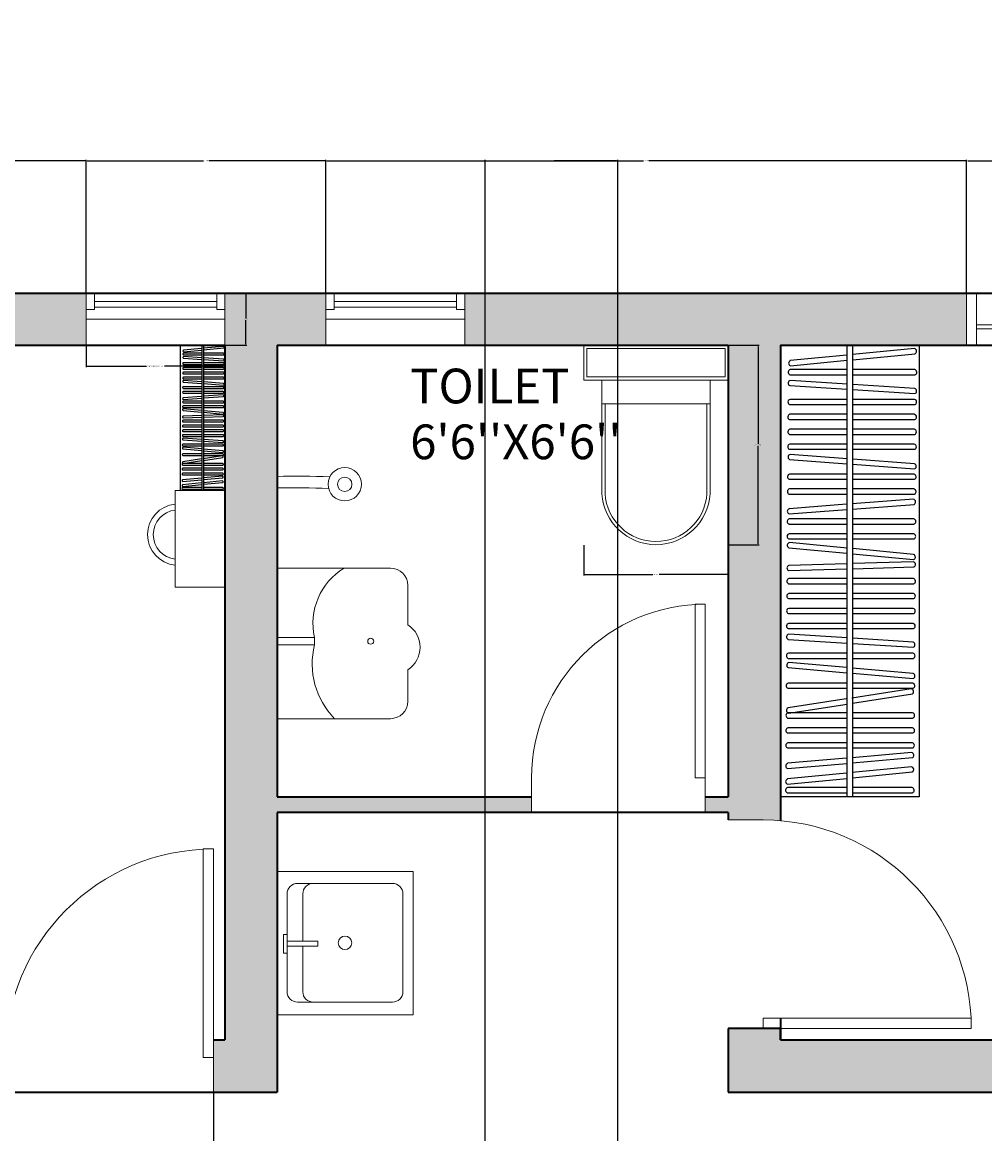
# Model space of a CAD drawing. Units: inches. Extents: x 1789 to 2841, y 3180 to 3702.
# Tile 6 of 14: x 2041 to 2208, y 3510 to 3702. Entities that reach past the tile are written whole.
import ezdxf

# ---------------------------------------------------------------- set-up
doc = ezdxf.new("R2010")
doc.units = ezdxf.units.IN
doc.header["$MEASUREMENT"] = 0
for name, color, linetype, lineweight in [('A-ANNO-DIMS', 2, 'Continuous', 18), ('A-AREA-IDEN', 7, 'Continuous', 18), ('A-FLOR-CASE', 34, 'Continuous', 25), ('A-FLOR-FIXT', 9, 'Continuous', 18), ('A-WALL', 40, 'Continuous', 35), ('A-WALL-PATT', 252, 'Continuous', 13), ('DORS', 70, 'Continuous', 18), ('FURNITURE', 34, 'Continuous', 18), ('WINDOWS', 130, 'Continuous', 18)]:
    doc.layers.add(name, color=color, linetype=linetype, lineweight=lineweight)
doc.styles.get("Standard").update_dxf_attribs({"font": 'arial.ttf'})
doc.dimstyles.get("Standard").update_dxf_attribs({"dimtxt": 0.18, "dimasz": 0.18, "dimexe": 0.18, "dimexo": 0.0625, "dimgap": 0.09, "dimtad": 0, "dimtih": 1, "dimtoh": 1, "dimdec": 0, "dimzin": 0, "dimdsep": 46, "dimlunit": 3, "dimtxsty": 'Standard', "dimcen": 0.09, "dimadec": 0, "dimazin": 0, "dimtfac": 1, "dimtdec": 0, "dimtofl": 0, "dimtmove": 0, "dimatfit": 3, "dimfxl": 1, "dimtolj": 1, "dimtzin": 0, "dimarcsym": 0})

# ---------------------------------------------------------------- blocks, each defined once
blk = doc.blocks.new('HY')
for p, q in [((2053.67, 3653.75), (2074.8, 3653.75)), ((2053.67, 3652.75), (2074.8, 3652.75)), ((2052.23, 3650.66), (2076.23, 3650.66))]:
    blk.add_line(p, q)
for points in [[(2076.23, 3646.16), (2052.23, 3646.16), (2052.23, 3655.16), (2076.23, 3655.16)], [(2052.23, 3655.16), (2053.67, 3655.16), (2053.67, 3652.35), (2052.23, 3652.35)], [(2076.23, 3655.16), (2074.8, 3655.16), (2074.8, 3652.35), (2076.23, 3652.35)]]:
    blk.add_lwpolyline(points, close=True)
blk = doc.blocks.new('HYJ')
for p, q in [((2236.02, 3650.77), (2262.74, 3650.77)), ((2206.12, 3649.67), (2234.3, 3649.67)), ((2206.12, 3649), (2234.3, 3649)), ((2236.02, 3650.11), (2262.74, 3650.11))]:
    blk.add_line(p, q)
for points in [[(2204.43, 3646.16), (2264.43, 3646.16), (2264.43, 3655.16), (2204.43, 3655.16)], [(2204.43, 3655.16), (2206.12, 3655.16), (2206.12, 3646.16), (2204.43, 3646.16)], [(2264.43, 3655.16), (2262.74, 3655.16), (2262.74, 3646.16), (2264.43, 3646.16)], [(2235.16, 3650.77), (2236.02, 3650.77), (2236.02, 3649.67), (2235.16, 3649.67)], [(2234.3, 3649.67), (2235.16, 3649.67), (2235.16, 3648.56), (2234.3, 3648.56)]]:
    blk.add_lwpolyline(points, close=True)
blk = doc.blocks.new('CUBOARD')
for p, q in [((2183.73, 3646.16), (2183.73, 3568.16)), ((2184.71, 3646.16), (2184.71, 3568.16))]:
    blk.add_line(p, q)
blk.add_lwpolyline([(2172.23, 3646.16), (2196.23, 3646.16), (2196.23, 3568.16), (2172.23, 3568.16)], close=True)
for points in [[(2183.69, 3644.46), (2173.95, 3643.51)], [(2195.39, 3645.6), (2184.67, 3644.55)], [(2184.76, 3643.66), (2195.54, 3644.71)], [(2195.78, 3645.16), (2195.78, 3645.18)], [(2173.97, 3642.61), (2183.78, 3643.57)], [(2173.86, 3641.08), (2183.73, 3641.08)], [(2183.73, 3641.98), (2173.93, 3641.98)], [(2195.47, 3641.98), (2184.71, 3641.98)], [(2184.71, 3641.08), (2195.53, 3641.08)], [(2195.82, 3641.5), (2195.82, 3641.53)], [(2173.84, 3639.19), (2183.7, 3638.57)], [(2183.76, 3639.46), (2173.96, 3640.08)], [(2195.45, 3638.71), (2184.74, 3639.4)], [(2183.73, 3636.82), (2173.9, 3636.82)], [(2184.68, 3638.5), (2195.46, 3637.81)], [(2195.43, 3636.82), (2184.71, 3636.82)], [(2195.77, 3638.22), (2195.78, 3638.24)], [(2173.83, 3635.92), (2183.73, 3635.92)], [(2184.71, 3635.92), (2195.5, 3635.92)], [(2195.78, 3636.35), (2195.78, 3636.37)], [(2173.81, 3633.34), (2183.73, 3633.34)], [(2183.73, 3634.24), (2173.88, 3634.24)], [(2195.42, 3634.24), (2184.71, 3634.24)], [(2184.71, 3633.34), (2195.48, 3633.34)], [(2195.77, 3633.77), (2195.77, 3633.79)], [(2183.73, 3631.66), (2173.86, 3631.66)], [(2195.4, 3631.66), (2184.71, 3631.66)], [(2195.75, 3631.19), (2195.75, 3631.21)], [(2173.8, 3630.76), (2183.73, 3630.76)], [(2183.73, 3629.08), (2173.85, 3629.08)], [(2184.71, 3630.76), (2195.47, 3630.76)], [(2195.38, 3629.08), (2184.71, 3629.08)], [(2173.78, 3628.19), (2183.73, 3628.19)], [(2183.8, 3626.57), (2173.93, 3627.31)], [(2184.71, 3628.19), (2195.45, 3628.19)], [(2195.73, 3628.61), (2195.73, 3628.63)], [(2173.79, 3626.43), (2183.74, 3625.68)], [(2184.71, 3625.61), (2195.4, 3624.81)], [(2195.4, 3625.7), (2184.78, 3626.5)], [(2195.72, 3625.21), (2195.72, 3625.23)], [(2183.73, 3623.92), (2173.81, 3623.92)], [(2195.35, 3623.92), (2184.71, 3623.92)], [(2195.7, 3623.45), (2195.7, 3623.48)], [(2173.75, 3623.03), (2183.73, 3623.03)], [(2183.73, 3621.34), (2173.8, 3621.34)], [(2184.71, 3623.03), (2195.42, 3623.03)], [(2195.33, 3621.34), (2184.71, 3621.34)], [(2173.73, 3620.45), (2183.73, 3620.45)], [(2195.22, 3619.57), (2184.65, 3618.76)], [(2184.71, 3620.45), (2195.4, 3620.45)], [(2195.68, 3620.87), (2195.68, 3620.9)], [(2183.67, 3618.69), (2173.75, 3617.93)], [(2173.75, 3617.03), (2183.74, 3617.8)], [(2184.71, 3617.87), (2195.35, 3618.68)], [(2195.6, 3619.13), (2195.6, 3619.15)], [(2183.73, 3616.19), (2173.77, 3616.19)], [(2195.3, 3616.19), (2184.71, 3616.19)], [(2195.65, 3615.71), (2195.65, 3615.74)], [(2173.7, 3615.29), (2183.73, 3615.29)], [(2184.71, 3615.29), (2195.37, 3615.29)], [(2173.68, 3612.71), (2183.73, 3612.71)], [(2183.73, 3613.61), (2173.75, 3613.61)], [(2183.78, 3611.12), (2173.82, 3612.07)], [(2195.28, 3613.61), (2184.71, 3613.61)], [(2184.71, 3612.71), (2195.35, 3612.71)], [(2195.63, 3613.14), (2195.63, 3613.16)], [(2173.67, 3611.18), (2183.69, 3610.23)], [(2184.67, 3610.14), (2195.24, 3609.13)], [(2195.26, 3610.03), (2184.75, 3611.03)], [(2183.72, 3608.42), (2173.71, 3608.13)], [(2195.23, 3608.76), (2184.7, 3608.45)], [(2195.56, 3609.53), (2195.57, 3609.55)], [(2195.6, 3608.3), (2195.6, 3608.32)], [(2173.66, 3607.23), (2183.75, 3607.53)], [(2184.73, 3607.55), (2195.33, 3607.87)], [(2173.63, 3604.98), (2183.73, 3604.98)], [(2183.73, 3605.87), (2173.7, 3605.87)], [(2195.23, 3605.87), (2184.71, 3605.87)], [(2184.71, 3604.98), (2195.3, 3604.98)], [(2195.58, 3605.4), (2195.58, 3605.42)], [(2173.61, 3602.4), (2183.73, 3602.4)], [(2183.73, 3603.29), (2173.68, 3603.29)], [(2195.22, 3603.29), (2184.71, 3603.29)], [(2184.71, 3602.4), (2195.28, 3602.4)], [(2195.57, 3602.82), (2195.57, 3602.84)], [(2183.73, 3600.71), (2173.67, 3600.71)], [(2195.2, 3600.71), (2184.71, 3600.71)], [(2195.55, 3600.24), (2195.55, 3600.27)], [(2173.6, 3599.82), (2183.73, 3599.82)], [(2184.71, 3599.82), (2195.27, 3599.82)], [(2173.58, 3597.24), (2183.73, 3597.24)], [(2183.73, 3598.13), (2173.65, 3598.13)], [(2195.18, 3598.13), (2184.71, 3598.13)], [(2184.71, 3597.24), (2195.25, 3597.24)], [(2195.53, 3597.66), (2195.53, 3597.69)], [(2173.56, 3595.36), (2183.71, 3594.72)], [(2183.77, 3595.62), (2173.68, 3596.25)], [(2184.69, 3594.66), (2195.19, 3594)], [(2195.18, 3594.9), (2184.74, 3595.55)], [(2183.73, 3592.98), (2173.62, 3592.98)], [(2195.15, 3592.98), (2184.71, 3592.98)], [(2195.5, 3594.4), (2195.5, 3594.43)], [(2195.5, 3592.5), (2195.5, 3592.53)], [(2173.55, 3592.08), (2183.73, 3592.08)], [(2183.73, 3590.49), (2173.72, 3591.37)], [(2184.71, 3592.08), (2195.22, 3592.08)], [(2173.57, 3590.49), (2183.74, 3589.59)], [(2195.17, 3589.47), (2184.71, 3590.4)], [(2184.71, 3589.5), (2195.16, 3588.58)], [(2195.48, 3588.97), (2195.48, 3589)], [(2173.51, 3586.92), (2183.73, 3586.92)], [(2183.73, 3587.82), (2173.58, 3587.82)], [(2194.84, 3586.83), (2184.58, 3585.23)], [(2195.12, 3587.82), (2184.71, 3587.82)], [(2184.71, 3586.92), (2195.19, 3586.92)], [(2195.47, 3587.35), (2195.47, 3587.37)], [(2183.61, 3585.08), (2173.56, 3583.51)], [(2184.71, 3584.34), (2195.04, 3585.95)], [(2195.26, 3586.41), (2195.25, 3586.44)], [(2173.63, 3582.62), (2183.75, 3584.19)], [(2173.48, 3581.77), (2183.73, 3581.77)], [(2183.73, 3582.66), (2173.55, 3582.66)], [(2195.08, 3582.66), (2184.71, 3582.66)], [(2184.71, 3581.77), (2195.15, 3581.77)], [(2195.43, 3582.19), (2195.43, 3582.21)], [(2173.46, 3579.19), (2183.73, 3579.19)], [(2183.73, 3580.08), (2173.53, 3580.08)], [(2195.07, 3580.08), (2184.71, 3580.08)], [(2184.71, 3579.19), (2195.14, 3579.19)], [(2195.42, 3579.61), (2195.42, 3579.63)], [(2183.73, 3577.5), (2173.52, 3577.5)], [(2195.05, 3577.5), (2184.71, 3577.5)], [(2173.45, 3576.61), (2183.73, 3576.61)], [(2194.92, 3575.81), (2184.64, 3574.92)], [(2184.71, 3576.61), (2195.12, 3576.61)], [(2195.31, 3575.37), (2195.31, 3575.4)], [(2195.4, 3577.03), (2195.4, 3577.05)], [(2183.66, 3574.84), (2173.46, 3573.95)], [(2173.47, 3573.05), (2183.74, 3573.94)], [(2194.88, 3573.34), (2184.63, 3572.34)], [(2184.71, 3574.03), (2195.06, 3574.93)], [(2183.65, 3572.24), (2173.45, 3571.25)], [(2184.71, 3571.45), (2195.04, 3572.46)], [(2195.28, 3572.91), (2195.27, 3572.93)], [(2173.47, 3570.35), (2183.74, 3571.35)], [(2183.73, 3569.77), (2173.47, 3569.77)], [(2195, 3569.77), (2184.71, 3569.77)], [(2173.4, 3568.87), (2183.73, 3568.87)], [(2184.71, 3568.87), (2195.07, 3568.87)], [(2195.35, 3569.29), (2195.35, 3569.32)]]:
    blk.add_lwpolyline(points)
for centre, start, end in [((2195.31, 3645.13), 7.0195, 80.386), ((2195.31, 3645.13), 299.464, 4.1032), ((2174.12, 3643.06), 110.7367, 251.6587), ((2174.06, 3641.52), 105.1753, 246.0974), ((2195.34, 3641.52), 1.4582, 74.8247), ((2195.34, 3641.52), 293.9026, 358.5418), ((2174.06, 3639.62), 101.5232, 242.4452), ((2195.3, 3638.26), 357.8061, 71.1726), ((2174.02, 3636.36), 105.1753, 246.0974), ((2195.31, 3636.36), 1.4582, 74.8247), ((2195.3, 3638.26), 290.2505, 354.8897), ((2195.31, 3636.36), 293.9026, 358.5418), ((2174.01, 3633.78), 105.1753, 246.0974), ((2195.29, 3633.78), 1.4582, 74.8247), ((2195.29, 3633.78), 293.9026, 358.5418), ((2173.99, 3631.2), 105.1753, 246.0974), ((2195.27, 3631.2), 1.4582, 74.8247), ((2195.27, 3631.2), 293.9026, 358.5418), ((2173.97, 3628.62), 105.1753, 246.0974), ((2195.26, 3628.62), 1.4582, 74.8247), ((2174.02, 3626.85), 100.888, 241.81), ((2195.26, 3628.62), 293.9026, 358.5418), ((2195.24, 3625.25), 357.1709, 70.5374), ((2195.24, 3625.25), 289.6153, 354.2545), ((2173.94, 3623.46), 105.1753, 246.0974), ((2195.22, 3623.46), 1.4582, 74.8247), ((2195.22, 3623.46), 293.9026, 358.5418), ((2173.92, 3620.88), 105.1753, 246.0974), ((2195.21, 3620.88), 1.4582, 74.8247), ((2195.13, 3619.1), 5.8369, 79.2034), ((2195.21, 3620.88), 293.9026, 358.5418), ((2173.9, 3617.48), 109.5541, 250.4761), ((2195.13, 3619.1), 298.2814, 2.9206), ((2173.89, 3615.73), 105.1753, 246.0974), ((2195.17, 3615.73), 1.4582, 74.8247), ((2195.17, 3615.73), 293.9026, 358.5418), ((2173.87, 3613.15), 105.1753, 246.0974), ((2173.9, 3611.6), 99.7479, 240.6699), ((2195.16, 3613.15), 1.4582, 74.8247), ((2195.16, 3613.15), 293.9026, 358.5418), ((2195.09, 3609.58), 356.0307, 69.3973), ((2173.84, 3607.67), 106.858, 247.78), ((2195.12, 3608.3), 3.1408, 76.5073), ((2195.09, 3609.58), 288.4752, 353.1144), ((2195.12, 3608.3), 295.5853, 0.2245), ((2173.82, 3605.41), 105.1753, 246.0974), ((2195.11, 3605.41), 1.4582, 74.8247), ((2195.11, 3605.41), 293.9026, 358.5418), ((2173.81, 3602.83), 105.1753, 246.0974), ((2195.09, 3602.83), 1.4582, 74.8247), ((2195.09, 3602.83), 293.9026, 358.5418), ((2173.79, 3600.25), 105.1753, 246.0974), ((2195.08, 3600.25), 1.4582, 74.8247), ((2195.08, 3600.25), 293.9026, 358.5418), ((2173.77, 3597.67), 105.1753, 246.0974), ((2195.06, 3597.67), 1.4582, 74.8247), ((2195.06, 3597.67), 293.9026, 358.5418), ((2173.78, 3595.78), 101.566, 242.4881), ((2195.02, 3594.44), 357.8489, 71.2154), ((2173.74, 3592.52), 105.1753, 246.0974), ((2195.03, 3592.52), 1.4582, 74.8247), ((2195.02, 3594.44), 290.2933, 354.9325), ((2173.8, 3590.9), 100.1162, 241.0382), ((2195.03, 3592.52), 293.9026, 358.5418), ((2195.01, 3589.03), 288.8435, 353.4827), ((2195.01, 3589.03), 356.399, 69.7655), ((2173.71, 3587.36), 105.1753, 246.0974), ((2194.79, 3586.35), 10.3063, 83.6728), ((2194.99, 3587.36), 1.4582, 74.8247), ((2194.99, 3587.36), 293.9026, 358.5418), ((2194.79, 3586.35), 302.7507, 7.3899), ((2173.75, 3583.08), 114.0234, 254.9455), ((2173.67, 3582.2), 105.1753, 246.0974), ((2194.96, 3582.2), 1.4582, 74.8247), ((2194.96, 3582.2), 293.9026, 358.5418), ((2173.66, 3579.62), 105.1753, 246.0974), ((2194.94, 3579.62), 1.4582, 74.8247), ((2194.94, 3579.62), 293.9026, 358.5418), ((2173.64, 3577.04), 105.1753, 246.0974), ((2194.93, 3577.04), 1.4582, 74.8247), ((2194.83, 3575.34), 6.4142, 79.7807), ((2194.83, 3575.34), 298.8587, 3.4979), ((2194.93, 3577.04), 293.9026, 358.5418), ((2173.63, 3573.5), 110.1314, 251.0534), ((2194.8, 3572.87), 7.0476, 80.4142), ((2194.8, 3572.87), 299.4921, 4.1313), ((2173.59, 3569.31), 105.1753, 246.0974), ((2173.62, 3570.8), 110.7648, 251.6868), ((2194.88, 3569.31), 1.4582, 74.8247), ((2194.88, 3569.31), 293.9026, 358.5418)]:
    blk.add_arc(centre, 0.476, start, end)
blk = doc.blocks.new('GT')
for p, q in [((2141.38, 3640.15), (2141.38, 3620.49)), ((2160.08, 3640.15), (2160.08, 3620.49)), ((2141.38, 3636.04), (2160.08, 3636.04)), ((2141.93, 3636.04), (2141.93, 3620.49)), ((2159.53, 3636.04), (2159.53, 3620.49))]:
    blk.add_line(p, q)
for points in [[(2163.23, 3646.16), (2138.23, 3646.16), (2138.23, 3640.15), (2163.23, 3640.15)], [(2162.68, 3645.61), (2138.78, 3645.61), (2138.78, 3640.7), (2162.68, 3640.7)]]:
    blk.add_lwpolyline(points, close=True)
for radius in [9.37, 8.82]:
    blk.add_arc((2150.73, 3621.09), radius, 183.6546, 356.3454)
blk = doc.blocks.new('KIKI')
blk.add_lwpolyline([(2076.23, 3621.09), (2067.63, 3621.09), (2067.63, 3604.37), (2076.23, 3604.37)], close=True)
for radius, start, end in [(5.28, 95.3029, 264.6971), (4.28, 96.5454, 263.4546)]:
    blk.add_arc((2068.12, 3613.45), radius, start, end)
blk = doc.blocks.new('*U9')
for p, q in [((0, 0), (0, -6)), ((36, 0), (36, -6))]:
    blk.add_line(p, q)
blk.add_lwpolyline([(0, 0), (0, 36), (1.75, 36), (1.75, 0)], close=True)
blk.add_arc((0, 0), 36, 0, 90)
blk = doc.blocks.new('*U10')
for p, q in [((0, 0), (0, -6)), ((30, 0), (30, -6))]:
    blk.add_line(p, q)
blk.add_lwpolyline([(0, 0), (0, 30), (1.75, 30), (1.75, 0)], close=True)
blk.add_arc((0, 0), 30, 0, 90)
blk = doc.blocks.new('TYTY')
for p, q in [((2104.84, 3607.68), (2085.23, 3607.68)), ((2085.23, 3607.68), (2085.23, 3581.66)), ((2107.84, 3597.9), (2107.84, 3604.68)), ((2107.84, 3584.66), (2107.84, 3590.13)), ((2085.23, 3581.66), (2104.84, 3581.66))]:
    blk.add_line(p, q)
blk.add_lwpolyline([(2085.23, 3595.66), (2091.71, 3595.66), (2091.71, 3594.41), (2085.23, 3594.41)], close=True)
blk.add_circle((2101.42, 3595.04), 0.517)
for centre, radius, start, end in [((2102.58, 3598.14), 11.14, 121.1396, 192.8397), ((2104.84, 3604.68), 3, 0, 90), ((2105.34, 3594.01), 4.62, 302.7804, 57.2196), ((2104.89, 3591.14), 13.58, 166.0641, 224.2681), ((2104.84, 3584.66), 3, 270, 0)]:
    blk.add_arc(centre, radius, start, end)
blk = doc.blocks.new('SINK')
for points in [[(2247.56, 3305.33), (2275.07, 3305.33), (2275.07, 3279.16), (2247.56, 3279.16)], [(2260.91, 3287.01), (2261.87, 3287.01), (2261.87, 3281.09), (2260.91, 3281.09)], [(2259.67, 3281.09), (2263.21, 3281.09), (2263.21, 3280.41), (2259.67, 3280.41)]]:
    blk.add_lwpolyline(points, close=True)
blk.add_lwpolyline([(2251.84, 3281.09), (2270.63, 3281.09, 0.414214), (2272.63, 3283.09), (2272.63, 3301.33, 0.414214), (2270.63, 3303.33), (2251.84, 3303.33, 0.414214), (2249.84, 3301.33), (2249.84, 3283.09, 0.414214)], format="xyb", close=True)
for points in [[(2249.84, 3301.33), (2249.84, 3286.11, 0.414214), (2251.84, 3284.11), (2260.91, 3284.11)], [(2261.87, 3284.11), (2270.63, 3284.11, 0.414214), (2272.63, 3286.11), (2272.63, 3301.33)]]:
    blk.add_lwpolyline(points, format="xyb")
blk.add_circle((2261.24, 3292.21), 1.3)
blk = doc.blocks.new('SOUW')
for radius in [2.88, 1.24]:
    blk.add_circle((2096.93, 3622.15), radius)
for radius, start in [(130.14, 87.3378), (128.14, 87.3891)]:
    blk.add_arc((2088.3, 3493.42), radius, start, 91.3578)
blk = doc.blocks.new('*D29')
at = {"layer": 'A-ANNO-DIMS', "color": 0, "lineweight": -2, "transparency": 16777216}
for p, q in [((2052.23, 3646.1), (2052.23, 3642.38)), ((2076.23, 3646.1), (2076.23, 3642.38)), ((2052.41, 3642.56), (2062.67, 3642.56)), ((2076.05, 3642.56), (2065.79, 3642.56))]:
    blk.add_line(p, q, dxfattribs=at)
at = {"layer": 'A-ANNO-DIMS', "color": 0, "transparency": 16777216}
for points in [[(2052.41, 3642.59), (2052.41, 3642.53), (2052.23, 3642.56)], [(2076.05, 3642.59), (2076.05, 3642.53), (2076.23, 3642.56)]]:
    blk.add_solid(points, dxfattribs=at)
at = {"layer": 'Defpoints', "color": 0, "transparency": 16777216}
for p in [(2052.23, 3646.16), (2076.23, 3646.16), (2076.23, 3642.56)]:
    blk.add_point(p, dxfattribs=at)
at = {"layer": 'A-ANNO-DIMS', "color": 0, "transparency": 16777216, "insert": (2064.23, 3642.56), "char_height": 0.18, "attachment_point": 5}
blk.add_mtext('\\A1;SMALL WINDOW 24 TYP.', dxfattribs=at)
blk = doc.blocks.new('*D30')
at = {"layer": 'A-ANNO-DIMS', "color": 0, "lineweight": -2, "transparency": 16777216}
for p, q in [((2076.3, 3655.16), (2080.01, 3655.16)), ((2079.83, 3654.98), (2079.83, 3650.84)), ((2079.83, 3646.34), (2079.83, 3650.48)), ((2076.3, 3646.16), (2080.01, 3646.16))]:
    blk.add_line(p, q, dxfattribs=at)
at = {"layer": 'A-ANNO-DIMS', "color": 0, "transparency": 16777216}
for points in [[(2079.8, 3654.98), (2079.86, 3654.98), (2079.83, 3655.16)], [(2079.8, 3646.34), (2079.86, 3646.34), (2079.83, 3646.16)]]:
    blk.add_solid(points, dxfattribs=at)
at = {"layer": 'Defpoints', "color": 0, "transparency": 16777216}
for p in [(2076.23, 3655.16), (2079.83, 3655.16), (2076.23, 3646.16)]:
    blk.add_point(p, dxfattribs=at)
at = {"layer": 'A-ANNO-DIMS', "color": 0, "transparency": 16777216, "insert": (2079.83, 3650.66), "char_height": 0.18, "attachment_point": 5}
blk.add_mtext('\\A1;9 TYP.', dxfattribs=at)
blk = doc.blocks.new('*D43')
at = {"layer": 'A-ANNO-DIMS', "color": 0, "lineweight": -2, "transparency": 16777216}
for p, q in [((2163.3, 3646.16), (2168.58, 3646.16)), ((2168.4, 3645.98), (2168.4, 3629.12)), ((2168.4, 3611.89), (2168.4, 3628.75)), ((2163.3, 3611.71), (2168.58, 3611.71))]:
    blk.add_line(p, q, dxfattribs=at)
at = {"layer": 'A-ANNO-DIMS', "color": 0, "transparency": 16777216}
for points in [[(2168.37, 3645.98), (2168.43, 3645.98), (2168.4, 3646.16)], [(2168.37, 3611.89), (2168.43, 3611.89), (2168.4, 3611.71)]]:
    blk.add_solid(points, dxfattribs=at)
at = {"layer": 'Defpoints', "color": 0, "transparency": 16777216}
for p in [(2163.23, 3646.16), (2168.4, 3646.16), (2163.23, 3611.71)]:
    blk.add_point(p, dxfattribs=at)
at = {"layer": 'A-ANNO-DIMS', "color": 0, "transparency": 16777216, "insert": (2168.4, 3628.94), "char_height": 0.18, "attachment_point": 5}
blk.add_mtext('\\A1;WC 34 TYP.', dxfattribs=at)
blk = doc.blocks.new('*D44')
at = {"layer": 'A-ANNO-DIMS', "color": 0, "lineweight": -2, "transparency": 16777216}
for p, q in [((2138.23, 3611.65), (2138.23, 3606.37)), ((2163.23, 3611.65), (2163.23, 3606.37)), ((2138.41, 3606.55), (2150.2, 3606.55)), ((2163.05, 3606.55), (2151.26, 3606.55))]:
    blk.add_line(p, q, dxfattribs=at)
at = {"layer": 'A-ANNO-DIMS', "color": 0, "transparency": 16777216}
for points in [[(2138.41, 3606.58), (2138.41, 3606.52), (2138.23, 3606.55)], [(2163.05, 3606.58), (2163.05, 3606.52), (2163.23, 3606.55)]]:
    blk.add_solid(points, dxfattribs=at)
at = {"layer": 'Defpoints', "color": 0, "transparency": 16777216}
for p in [(2138.23, 3611.71), (2163.23, 3611.71), (2163.23, 3606.55)]:
    blk.add_point(p, dxfattribs=at)
at = {"layer": 'A-ANNO-DIMS', "color": 0, "transparency": 16777216, "insert": (2150.73, 3606.55), "char_height": 0.18, "attachment_point": 5}
blk.add_mtext('\\A1;25 TYP.', dxfattribs=at)
blk = doc.blocks.new('*D82')
at = {"layer": 'A-ANNO-DIMS', "color": 0, "lineweight": -2, "transparency": 16777216}
for p, q in [((1959.23, 3655.22), (1959.23, 3678.19)), ((1959.41, 3678.01), (2005.51, 3678.01)), ((2052.05, 3678.01), (2005.95, 3678.01)), ((2052.23, 3655.22), (2052.23, 3678.19))]:
    blk.add_line(p, q, dxfattribs=at)
at = {"layer": 'A-ANNO-DIMS', "color": 0, "transparency": 16777216}
for points in [[(1959.41, 3678.04), (1959.41, 3677.98), (1959.23, 3678.01)], [(2052.05, 3678.04), (2052.05, 3677.98), (2052.23, 3678.01)]]:
    blk.add_solid(points, dxfattribs=at)
at = {"layer": 'Defpoints', "color": 0, "transparency": 16777216}
for p in [(2052.23, 3678.01), (1959.23, 3655.16), (2052.23, 3655.16)]:
    blk.add_point(p, dxfattribs=at)
at = {"layer": 'A-ANNO-DIMS', "color": 0, "transparency": 16777216, "insert": (2005.73, 3678.01), "char_height": 0.18, "attachment_point": 5}
blk.add_mtext('\\A1;93', dxfattribs=at)
blk = doc.blocks.new('*D83')
at = {"layer": 'A-ANNO-DIMS', "color": 0, "lineweight": -2, "transparency": 16777216}
for p, q in [((2052.23, 3655.22), (2052.23, 3678.19)), ((2052.41, 3678.01), (2072.49, 3678.01)), ((2093.5, 3678.01), (2073.42, 3678.01)), ((2093.68, 3655.22), (2093.68, 3678.19))]:
    blk.add_line(p, q, dxfattribs=at)
at = {"layer": 'A-ANNO-DIMS', "color": 0, "transparency": 16777216}
for points in [[(2052.41, 3678.04), (2052.41, 3677.98), (2052.23, 3678.01)], [(2093.5, 3678.04), (2093.5, 3677.98), (2093.68, 3678.01)]]:
    blk.add_solid(points, dxfattribs=at)
at = {"layer": 'Defpoints', "color": 0, "transparency": 16777216}
for p in [(2093.68, 3678.01), (2052.23, 3655.16), (2093.68, 3655.16)]:
    blk.add_point(p, dxfattribs=at)
at = {"layer": 'A-ANNO-DIMS', "color": 0, "transparency": 16777216, "insert": (2072.96, 3678.01), "char_height": 0.18, "attachment_point": 5}
blk.add_mtext('\\A1;41.445', dxfattribs=at)
blk = doc.blocks.new('*D84')
at = {"layer": 'A-ANNO-DIMS', "color": 0, "lineweight": -2, "transparency": 16777216}
for p, q in [((2093.68, 3655.22), (2093.68, 3678.19)), ((2093.86, 3678.01), (2148.6, 3678.01)), ((2204.25, 3678.01), (2149.51, 3678.01)), ((2204.43, 3655.22), (2204.43, 3678.19))]:
    blk.add_line(p, q, dxfattribs=at)
at = {"layer": 'A-ANNO-DIMS', "color": 0, "transparency": 16777216}
for points in [[(2093.86, 3678.04), (2093.86, 3677.98), (2093.68, 3678.01)], [(2204.25, 3678.04), (2204.25, 3677.98), (2204.43, 3678.01)]]:
    blk.add_solid(points, dxfattribs=at)
at = {"layer": 'Defpoints', "color": 0, "transparency": 16777216}
for p in [(2204.43, 3678.01), (2093.68, 3655.16), (2204.43, 3655.16)]:
    blk.add_point(p, dxfattribs=at)
at = {"layer": 'A-ANNO-DIMS', "color": 0, "transparency": 16777216, "insert": (2149.06, 3678.01), "char_height": 0.18, "attachment_point": 5}
blk.add_mtext('\\A1;110.75', dxfattribs=at)
blk = doc.blocks.new('*D85')
at = {"layer": 'A-ANNO-DIMS', "color": 0, "lineweight": -2, "transparency": 16777216}
for p, q in [((2204.43, 3655.22), (2204.43, 3678.19)), ((2204.61, 3678.01), (2264.45, 3678.01)), ((2325.05, 3678.01), (2265.22, 3678.01)), ((2325.23, 3655.22), (2325.23, 3678.19))]:
    blk.add_line(p, q, dxfattribs=at)
at = {"layer": 'A-ANNO-DIMS', "color": 0, "transparency": 16777216}
for points in [[(2204.61, 3678.04), (2204.61, 3677.98), (2204.43, 3678.01)], [(2325.05, 3678.04), (2325.05, 3677.98), (2325.23, 3678.01)]]:
    blk.add_solid(points, dxfattribs=at)
at = {"layer": 'Defpoints', "color": 0, "transparency": 16777216}
for p in [(2325.23, 3678.01), (2204.43, 3655.16), (2325.23, 3655.16)]:
    blk.add_point(p, dxfattribs=at)
at = {"layer": 'A-ANNO-DIMS', "color": 0, "transparency": 16777216, "insert": (2264.83, 3678.01), "char_height": 0.18, "attachment_point": 5}
blk.add_mtext('\\A1;120.8', dxfattribs=at)
blk = doc.blocks.new('*D90')
at = {"layer": 'A-ANNO-DIMS', "color": 0, "lineweight": -2, "transparency": 16777216}
for p, q in [((2038.23, 3517.1), (2038.23, 3180.13)), ((2074.23, 3517.1), (2074.23, 3180.13)), ((2038.41, 3180.31), (2056.01, 3180.31)), ((2074.05, 3180.31), (2056.45, 3180.31))]:
    blk.add_line(p, q, dxfattribs=at)
at = {"layer": 'A-ANNO-DIMS', "color": 0, "transparency": 16777216}
for points in [[(2038.41, 3180.34), (2038.41, 3180.28), (2038.23, 3180.31)], [(2074.05, 3180.34), (2074.05, 3180.28), (2074.23, 3180.31)]]:
    blk.add_solid(points, dxfattribs=at)
at = {"layer": 'Defpoints', "color": 0, "transparency": 16777216}
for p in [(2038.23, 3517.16), (2074.23, 3517.16), (2074.23, 3180.31)]:
    blk.add_point(p, dxfattribs=at)
at = {"layer": 'A-ANNO-DIMS', "color": 0, "transparency": 16777216, "insert": (2056.23, 3180.31), "char_height": 0.18, "attachment_point": 5}
blk.add_mtext('\\A1;36', dxfattribs=at)
blk = doc.blocks.new('*D91')
at = {"layer": 'A-ANNO-DIMS', "color": 0, "lineweight": -2, "transparency": 16777216}
for p, q in [((2121.23, 3385.22), (2121.23, 3678.19)), ((2121.41, 3678.01), (2132.21, 3678.01)), ((2143.93, 3678.01), (2133.14, 3678.01)), ((2144.11, 3385.22), (2144.11, 3678.19))]:
    blk.add_line(p, q, dxfattribs=at)
at = {"layer": 'A-ANNO-DIMS', "color": 0, "transparency": 16777216}
for points in [[(2121.41, 3678.04), (2121.41, 3677.98), (2121.23, 3678.01)], [(2143.93, 3678.04), (2143.93, 3677.98), (2144.11, 3678.01)]]:
    blk.add_solid(points, dxfattribs=at)
at = {"layer": 'Defpoints', "color": 0, "transparency": 16777216}
for p in [(2144.11, 3678.01), (2121.23, 3385.16), (2144.11, 3385.16)]:
    blk.add_point(p, dxfattribs=at)
at = {"layer": 'A-ANNO-DIMS', "color": 0, "transparency": 16777216, "insert": (2132.67, 3678.01), "char_height": 0.18, "attachment_point": 5}
blk.add_mtext('\\A1;22.875', dxfattribs=at)
blk = doc.blocks.new('*D116')
at = {"layer": 'A-ANNO-DIMS', "color": 0, "lineweight": -2, "transparency": 16777216}
for p, q in [((1789.65, 3701.85), (1789.83, 3701.85)), ((1789.83, 3701.85), (1945.65, 3528.3)), ((2205.56, 3238.68), (2205.74, 3238.68)), ((2205.65, 3238.59), (2205.65, 3238.77))]:
    blk.add_line(p, q, dxfattribs=at)
at = {"layer": 'A-ANNO-DIMS', "color": 0, "transparency": 16777216}
blk.add_solid([(1945.67, 3528.32), (1945.62, 3528.28), (1945.77, 3528.16)], dxfattribs=at)
at = {"layer": 'Defpoints', "color": 0, "transparency": 16777216}
for p in [(1945.77, 3528.16), (2205.65, 3238.68)]:
    blk.add_point(p, dxfattribs=at)
at = {"layer": 'A-ANNO-DIMS', "color": 0, "transparency": 16777216, "insert": (1789.28, 3701.85), "char_height": 0.18, "attachment_point": 5}
blk.add_mtext('\\A1;R389', dxfattribs=at)

msp = doc.modelspace()

# ---------------------------------------------------------------- hatches: boundary and pattern name
at = {"layer": 'A-WALL-PATT'}
h = msp.add_hatch(color=256, dxfattribs=at)
h.dxf.hatch_style = 1
h.paths.add_polyline_path([(2052.2333, 3646.1608), (2052.2333, 3655.1608), (1959.2333, 3655.1608), (1959.2333, 3622.3936), (1968.2333, 3622.3936), (1968.2333, 3646.1608)])
h.paths.add_polyline_path([(2163.2333, 3646.1608), (2163.2333, 3640.1475), (2163.2333, 3568.1608), (2159.2333, 3568.1608), (2159.2333, 3565.4274), (2163.2333, 3565.4274), (2163.2333, 3564.1608), (2169.2333, 3564.1608, -0.02086055), (2172.2333, 3564.0356), (2172.2333, 3646.1608), (2196.2333, 3646.1608), (2204.4325, 3646.1608), (2204.4325, 3655.1608), (2117.6786, 3655.1608), (2117.6786, 3646.1608)])
h.paths.add_polyline_path([(2085.2333, 3646.1608), (2093.6786, 3646.1608), (2093.6786, 3655.1608), (2076.2333, 3655.1608), (2076.2333, 3646.1608), (2076.2333, 3621.0865), (2076.2333, 3526.1608), (2074.2333, 3526.1608), (2074.2333, 3523.1608), (2074.2333, 3517.1608), (2085.2333, 3517.1608), (2085.2333, 3565.4274), (2129.2333, 3565.4274), (2129.2333, 3568.1608), (2085.2333, 3568.1608)])
h.paths.add_polyline_path([(2172.2333, 3526.1608), (2172.2333, 3528.1608), (2163.2333, 3528.1608), (2163.2333, 3517.1608), (2316.2333, 3517.1608), (2316.2333, 3513.1608), (2319.2333, 3513.1608), (2325.2333, 3513.1608), (2325.2333, 3584.2279), (2316.2333, 3584.2279), (2316.2333, 3526.1608)])
h.paths.add_polyline_path([(2325.2333, 3655.1608), (2264.4325, 3655.1608), (2264.4325, 3646.1608), (2316.2333, 3646.1608), (2316.2333, 3633.8369), (2316.2333, 3620.2279), (2325.2333, 3620.2279)])

# ---------------------------------------------------------------- linework, layer by layer
at = {"layer": 'A-WALL'}
for p, q in [((1959.2333, 3655.1608), (2325.2333, 3655.1608)), ((1968.2333, 3646.1608), (2076.2333, 3646.1608)), ((2076.2333, 3646.1608), (2076.2333, 3526.1608)), ((2085.2333, 3646.1608), (2085.2333, 3568.1608)), ((2085.2333, 3646.1608), (2163.2333, 3646.1608)), ((2163.2333, 3646.1608), (2163.2333, 3568.1608)), ((2172.2333, 3646.1608), (2172.2333, 3564.0356)), ((2172.2333, 3646.1608), (2316.2333, 3646.1608)), ((2085.2333, 3568.1608), (2129.2333, 3568.1608)), ((2159.2333, 3568.1608), (2163.2333, 3568.1608)), ((2163.2333, 3565.4274), (2085.2333, 3565.4274)), ((2085.2333, 3565.4274), (2085.2333, 3517.1608)), ((2163.2333, 3565.4274), (2163.2333, 3564.1608)), ((2172.2333, 3529.9108), (2172.2333, 3526.1608)), ((2172.2333, 3528.1608), (2163.2333, 3528.1608)), ((2163.2333, 3528.1608), (2163.2333, 3517.1608)), ((2172.2333, 3526.1608), (2172.2333, 3528.1608)), ((2074.2333, 3526.1608), (2076.2333, 3526.1608)), ((2172.2333, 3526.1608), (2316.2333, 3526.1608)), ((1959.2333, 3517.1608), (2085.2333, 3517.1608)), ((2163.2333, 3517.1608), (2316.2333, 3517.1608))]:
    msp.add_line(p, q, dxfattribs=at)

# ---------------------------------------------------------------- block references
at = {"layer": 'A-FLOR-CASE', "xscale": 0.3214652351977254, "yscale": 0.3214652351977254, "zscale": 0.3214652351977254}
msp.add_blockref('CUBOARD', (1370.2207, 2474.0469), dxfattribs=at)
at = {"layer": 'A-FLOR-CASE'}
msp.add_blockref('CUBOARD', (0, 0), dxfattribs=at)
at = {"layer": 'A-FLOR-FIXT'}
for name in ['GT', 'SOUW', 'TYTY']:
    msp.add_blockref(name, (0, 0), dxfattribs=at)
at = {"layer": 'A-FLOR-FIXT', "xscale": 0.8998033160254596, "yscale": 0.8998033160254596, "zscale": 0.8998033160254596, "rotation": 270}
msp.add_blockref('SINK', (-865.3664, 5577.618), dxfattribs=at)
at = {"layer": 'DORS', "xscale": -1}
for name, p in [('*U10', (2159.2333, 3571.4274)), ('*U9', (2074.2333, 3523.1608))]:
    msp.add_blockref(name, p, dxfattribs=at)
at = {"layer": 'DORS', "xscale": -1, "rotation": 270}
msp.add_blockref('*U9', (2169.2333, 3528.1608), dxfattribs=at)
at = {"layer": 'FURNITURE'}
msp.add_blockref('KIKI', (0, 0), dxfattribs=at)
at = {"layer": 'WINDOWS'}
for name, p in [('HY', (0, 0)), ('HY', (41.4453, 0)), ('HYJ', (0, 0))]:
    msp.add_blockref(name, p, dxfattribs=at)

# ---------------------------------------------------------------- texts
at = {"layer": 'A-ANNO-DIMS'}
msp.add_text("6'6''X6'6''", height=6, dxfattribs=at).set_placement((2108.2402, 3626.4874))
at = {"layer": 'A-AREA-IDEN'}
msp.add_text('TOILET', height=6, dxfattribs=at).set_placement((2108.2402, 3636.1259))

# ---------------------------------------------------------------- dimensions: what is measured, and where the dimension line sits
at = {"layer": 'A-ANNO-DIMS'}
dim = msp.add_radius_dim(center=(2205.6545, 3238.6823), mpoint=(1945.766, 3528.162), dimstyle='Standard', override={"dimdec": 0, "dimlfac": 1, "dimrnd": 0, "dimzin": 0, "dimdsep": 46, "dimlunit": 2}, dxfattribs=at)
dim.commit()
dim.dimension.update_dxf_attribs({"geometry": '*D116', "text_midpoint": (1789.2778, 3701.8498), "dimtype": 164})
for base, p1, p2, override, picture, middle in [((2052.2333, 3678.0108), (1959.2333, 3655.1608), (2052.2333, 3655.1608), {"dimdec": 0, "dimlfac": 1, "dimrnd": 0, "dimzin": 0, "dimdsep": 46, "dimlunit": 2}, '*D82', (2005.7333, 3678.0108)), ((2093.6786, 3678.0108), (2052.2333, 3655.1608), (2093.6786, 3655.1608), {"dimdec": 3, "dimlfac": 1, "dimrnd": 0, "dimzin": 0, "dimdsep": 46, "dimlunit": 2}, '*D83', (2072.956, 3678.0108)), ((2204.4325, 3678.0108), (2093.6786, 3655.1608), (2204.4325, 3655.1608), {"dimdec": 2, "dimlfac": 1, "dimrnd": 0, "dimzin": 0, "dimdsep": 46, "dimlunit": 2}, '*D84', (2149.0556, 3678.0108)), ((2144.1086, 3678.0108), (2121.2333, 3385.1608), (2144.1086, 3385.1608), {"dimdec": 3, "dimlfac": 1, "dimrnd": 0, "dimzin": 0, "dimdsep": 46, "dimlunit": 2}, '*D91', (2132.671, 3678.0108)), ((2325.2333, 3678.0108), (2204.4325, 3655.1608), (2325.2333, 3655.1608), {"dimdec": 1, "dimlfac": 1, "dimrnd": 0, "dimzin": 0, "dimdsep": 46, "dimlunit": 2}, '*D85', (2264.8329, 3678.0108)), ((2074.2333, 3180.3108), (2038.2333, 3517.1608), (2074.2333, 3517.1608), {"dimdec": 0, "dimlfac": 1, "dimrnd": 0, "dimzin": 0, "dimdsep": 46, "dimlunit": 2}, '*D90', (2056.2333, 3180.3108))]:
    dim = msp.add_linear_dim(base=base, p1=p1, p2=p2, dimstyle='Standard', override=override, dxfattribs=at)
    dim.commit()
    dim.dimension.update_dxf_attribs({"geometry": picture, "text_midpoint": middle})
for base, p1, p2, text, picture, middle in [((2079.8333, 3655.1608), (2076.2333, 3646.1608), (2076.2333, 3655.1608), '<> TYP.', '*D30', (2079.8333, 3650.6608)), ((2168.4003, 3646.1608), (2163.2333, 3611.7145), (2163.2333, 3646.1608), 'WC <> TYP.', '*D43', (2168.4003, 3628.9376))]:
    dim = msp.add_linear_dim(base=base, p1=p1, p2=p2, angle=90, text=text, dimstyle='Standard', override={"dimdec": 0, "dimlfac": 1, "dimrnd": 0, "dimzin": 0, "dimdsep": 46, "dimlunit": 2}, dxfattribs=at)
    dim.commit()
    dim.dimension.update_dxf_attribs({"geometry": picture, "text_midpoint": middle})
for base, p1, p2, text, picture, middle in [((2076.2333, 3642.5608), (2052.2333, 3646.1608), (2076.2333, 3646.1608), 'SMALL WINDOW <> TYP.', '*D29', (2064.2333, 3642.5608)), ((2163.2333, 3606.5476), (2138.2295, 3611.7145), (2163.2333, 3611.7145), '<> TYP.', '*D44', (2150.7314, 3606.5476))]:
    dim = msp.add_linear_dim(base=base, p1=p1, p2=p2, text=text, dimstyle='Standard', override={"dimdec": 0, "dimlfac": 1, "dimrnd": 0, "dimzin": 0, "dimdsep": 46, "dimlunit": 2}, dxfattribs=at)
    dim.commit()
    dim.dimension.update_dxf_attribs({"geometry": picture, "text_midpoint": middle})

doc.saveas('drawing.dxf')
